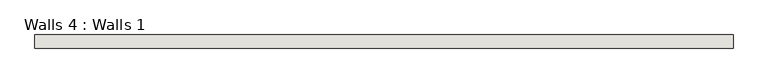
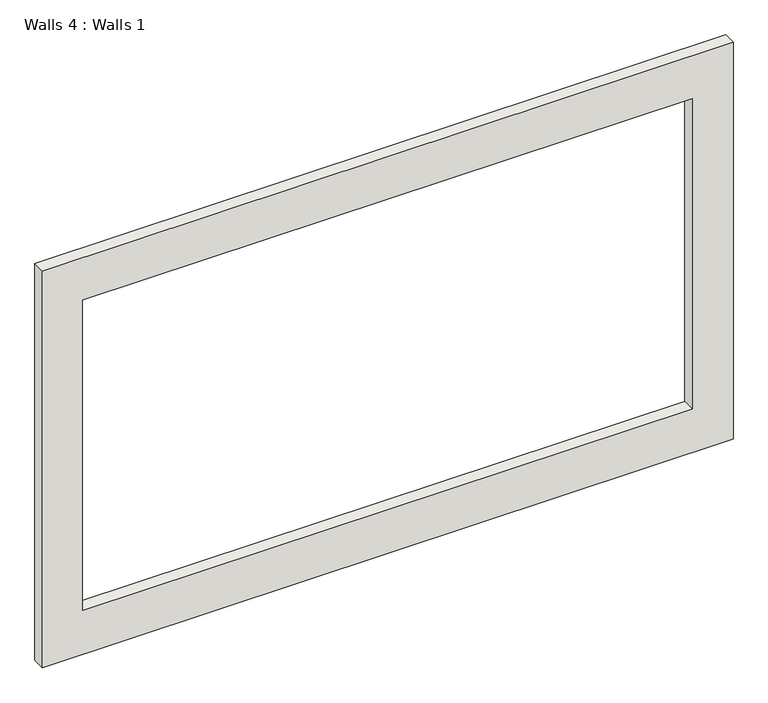
"""IFC4 building model written with IfcOpenShell, lengths in millimetres: wall geometry, Walls 4 : Walls 1."""

from ifc_helpers import new_model, si_unit, frame, origin, place, context, project, spatial, polyline, outline, extrude, source, transform, mapped, element, save


def walls_4_walls_1_cdf310b5(model_context):
    return source(origin(), model_context, "Body", "SweptSolid", [
        extrude(outline(polyline([(10319.3693979, 1712.6958607), (10319.3693979, -878.1041393), (8744.5693979, -878.1041393), (8744.5693979, 1712.6958607), (10319.3693979, 1712.6958607)]), holes=[polyline([(10149.624337, 1560.0533085), (8918.7422066, 1560.0533085), (8918.7422066, -725.9466915), (10149.624337, -725.9466915), (10149.624337, 1560.0533085)])]), frame((0.0, -4192.4325754, 0.0), z_axis=(0.0, 1.0, 0.0), x_axis=(0.0, 0.0, 1.0)), (0.0, 0.0, 1.0), 48.6357193),
    ])


if __name__ == "__main__":
    model = new_model("IFC4")
    model_context = context("Model", 3, world=origin())
    ifc_project = project(units=[si_unit("LENGTHUNIT", "METRE", prefix="MILLI")], contexts=[model_context])
    site = spatial("IfcSite", under=ifc_project)
    building = spatial("IfcBuilding", under=site)
    placement = place(None, origin())
    walls_4_walls_1_shape = walls_4_walls_1_cdf310b5(model_context)
    element("IfcWall", 1, ObjectType="Walls 4 : Walls 1", at=placement, inside=building, context=model_context, shape_type="MappedRepresentation", body=[
        mapped(walls_4_walls_1_shape, transform((0.0, 0.0, 0.0), x_axis=(1.0, 0.0, 0.0), y_axis=(0.0, 1.0, 0.0), z_axis=(0.0, 0.0, 1.0))),
    ])
    save(model, "model.ifc")

# Revit data of these elements
# Element 1 (IfcWall, "Walls 4 : Walls 1")
#   Materials on its faces: "Default Wall"
# Materials
#   "Default Wall": colour RGB 128 128 128, transparency 0
